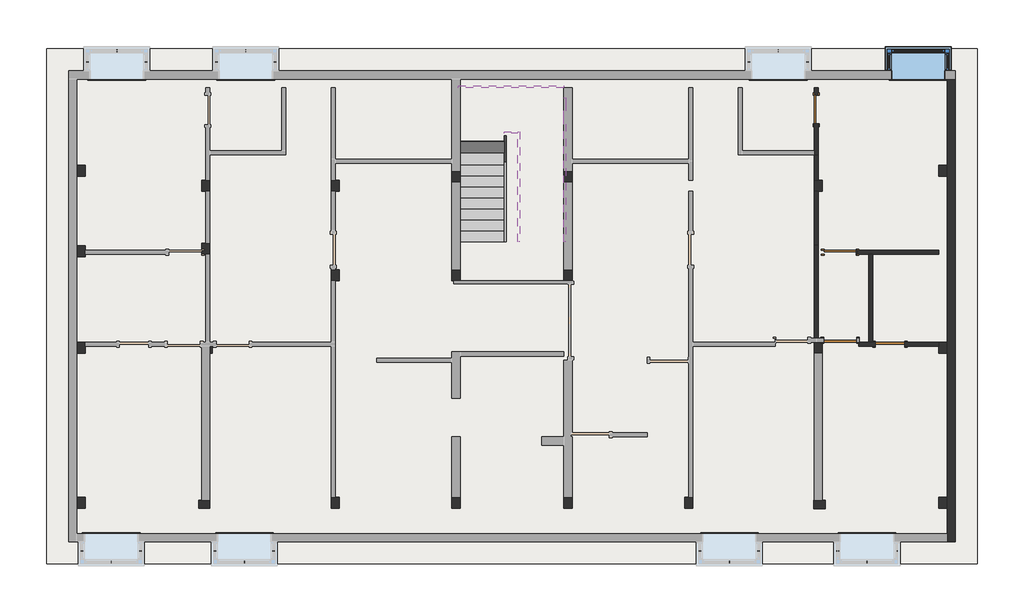
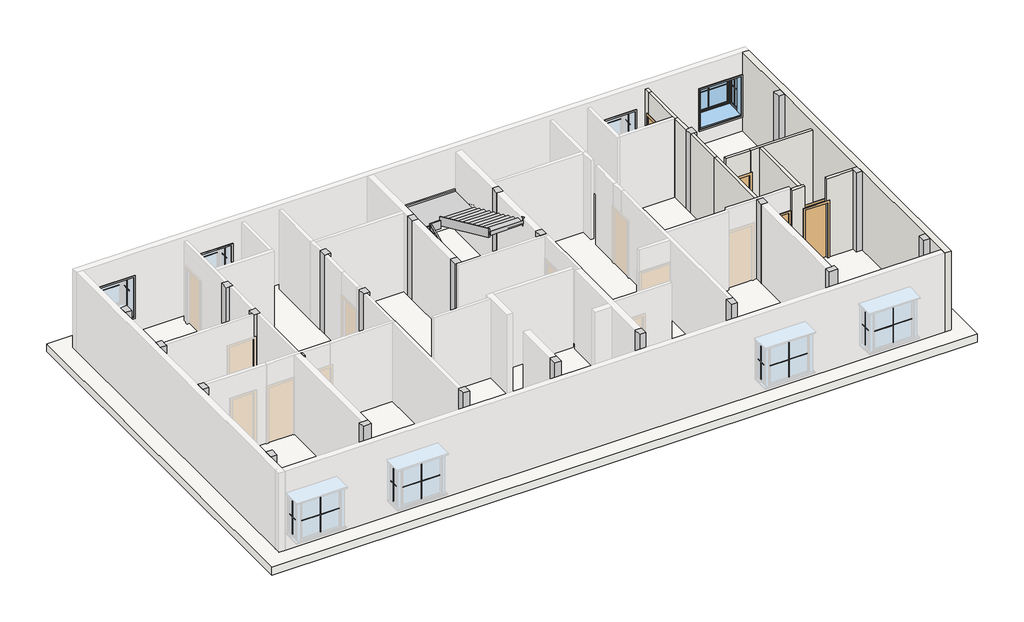
# One storey, part 2 of 2: 32 proxies, 24 columns, 11 walls, 6 members, 4 doors, 1 slab, 1 stair flight, 1 window.
"""IFC4 building model written with IfcOpenShell, lengths in millimetres."""

from ifc_helpers import new_model, si_unit, frame, origin, place, context, project, spatial, polyline, outline, extrude, faceted_brep, transform, mapped, element, save
from components import m_muntin_pattern_2x2_m_muntin_pattern_2x2_c1fd4460, m_muntin_pattern_2x2_m_muntin_pattern_2x2_777b163a, m_trim_window_interior_flat_picture_frame_44e8afef, column_efe9d5a4, door_1991e9a2, door_a431d384, door_82def9da, m_door_single_panel_3_x7_f8176753, stair_flight_1c36809e, window_19bbd869

model = new_model("IFC4")

# Units and contexts
model_context = context("Model", 3, world=origin())
ifc_project = project(units=[si_unit("LENGTHUNIT", "METRE", prefix="MILLI")], contexts=[model_context])

# Site, building, storey
site = spatial("IfcSite", under=ifc_project)
building = spatial("IfcBuilding", under=site)
storey = spatial("IfcBuildingStorey", under=building, Elevation=16002.0)

# Proxies
placement = place(None, origin())
m_muntin_pattern_2x2_m_muntin_pattern_2x2_shape = m_muntin_pattern_2x2_m_muntin_pattern_2x2_c1fd4460(model_context)
element("IfcBuildingElementProxy", 1, Name="M_Muntin Pattern_2x2 : M_Muntin Pattern_2x2", ObjectType="M_Muntin Pattern_2x2 : M_Muntin Pattern_2x2", at=placement, inside=storey, context=model_context, shape_type="MappedRepresentation", body=[
    mapped(m_muntin_pattern_2x2_m_muntin_pattern_2x2_shape, transform((-11500.7987957, -5499.9182661, 16722.65), x_axis=(-1.0, 0.0, 0.0), y_axis=(0.0, -1.0, 0.0), z_axis=(0.0, 0.0, 1.0))),
])
element("IfcBuildingElementProxy", 2, Name="M_Muntin Pattern_2x2 : M_Muntin Pattern_2x2", ObjectType="M_Muntin Pattern_2x2 : M_Muntin Pattern_2x2", at=placement, inside=storey, context=model_context, shape_type="MappedRepresentation", body=[
    mapped(m_muntin_pattern_2x2_m_muntin_pattern_2x2_shape, transform((-7819.250543, -5499.9182661, 16722.65), x_axis=(-1.0, 0.0, 0.0), y_axis=(0.0, -1.0, 0.0), z_axis=(0.0, 0.0, 1.0))),
])
element("IfcBuildingElementProxy", 3, Name="M_Muntin Pattern_2x2 : M_Muntin Pattern_2x2", ObjectType="M_Muntin Pattern_2x2 : M_Muntin Pattern_2x2", at=placement, inside=storey, context=model_context, shape_type="MappedRepresentation", body=[
    mapped(m_muntin_pattern_2x2_m_muntin_pattern_2x2_shape, transform((5599.7512082, -5499.9182661, 16722.65), x_axis=(-1.0, 0.0, 0.0), y_axis=(0.0, -1.0, 0.0), z_axis=(0.0, 0.0, 1.0))),
])
element("IfcBuildingElementProxy", 4, Name="M_Muntin Pattern_2x2 : M_Muntin Pattern_2x2", ObjectType="M_Muntin Pattern_2x2 : M_Muntin Pattern_2x2", at=placement, inside=storey, context=model_context, shape_type="MappedRepresentation", body=[
    mapped(m_muntin_pattern_2x2_m_muntin_pattern_2x2_shape, transform((9408.6146942, -5499.9182662, 16722.65), x_axis=(-1.0, 0.0, 0.0), y_axis=(0.0, -1.0, 0.0), z_axis=(0.0, 0.0, 1.0))),
])
element("IfcBuildingElementProxy", 5, Name="M_Muntin Pattern_2x2 : M_Muntin Pattern_2x2", ObjectType="M_Muntin Pattern_2x2 : M_Muntin Pattern_2x2", at=placement, inside=storey, context=model_context, shape_type="MappedRepresentation", body=[
    mapped(m_muntin_pattern_2x2_m_muntin_pattern_2x2_shape, transform((-11348.3987957, 8647.7317329, 16722.65), x_axis=(1.0, 0.0, 0.0), y_axis=(0.0, 1.0, 0.0), z_axis=(0.0, 0.0, 1.0))),
])
element("IfcBuildingElementProxy", 6, Name="M_Muntin Pattern_2x2 : M_Muntin Pattern_2x2", ObjectType="M_Muntin Pattern_2x2 : M_Muntin Pattern_2x2", at=placement, inside=storey, context=model_context, shape_type="MappedRepresentation", body=[
    mapped(m_muntin_pattern_2x2_m_muntin_pattern_2x2_shape, transform((-7779.6987993, 8647.7317329, 16722.65), x_axis=(1.0, 0.0, 0.0), y_axis=(0.0, 1.0, 0.0), z_axis=(0.0, 0.0, 1.0))),
])
element("IfcBuildingElementProxy", 7, Name="M_Muntin Pattern_2x2 : M_Muntin Pattern_2x2", ObjectType="M_Muntin Pattern_2x2 : M_Muntin Pattern_2x2", at=placement, inside=storey, context=model_context, shape_type="MappedRepresentation", body=[
    mapped(m_muntin_pattern_2x2_m_muntin_pattern_2x2_shape, transform((6952.301208, 8647.7317329, 16722.65), x_axis=(1.0, 0.0, 0.0), y_axis=(0.0, 1.0, 0.0), z_axis=(0.0, 0.0, 1.0))),
])
element("IfcBuildingElementProxy", 8, Name="M_Muntin Pattern_2x2 : M_Muntin Pattern_2x2", ObjectType="M_Muntin Pattern_2x2 : M_Muntin Pattern_2x2", at=placement, inside=storey, context=model_context, shape_type="MappedRepresentation", body=[
    mapped(m_muntin_pattern_2x2_m_muntin_pattern_2x2_shape, transform((10825.8012075, 8647.7317329, 16722.65), x_axis=(1.0, 0.0, 0.0), y_axis=(0.0, 1.0, 0.0), z_axis=(0.0, 0.0, 1.0))),
])
m_muntin_pattern_2x2_m_muntin_pattern_2x2_2_shape = m_muntin_pattern_2x2_m_muntin_pattern_2x2_777b163a(model_context)
element("IfcBuildingElementProxy", 9, Name="M_Muntin Pattern_2x2 : M_Muntin Pattern_2x2", ObjectType="M_Muntin Pattern_2x2 : M_Muntin Pattern_2x2", at=placement, inside=storey, context=model_context, shape_type="MappedRepresentation", body=[
    mapped(m_muntin_pattern_2x2_m_muntin_pattern_2x2_2_shape, transform((-10690.4737957, -5190.3932661, 16722.65), x_axis=(0.0, 1.0, 0.0), y_axis=(-1.0, 0.0, 0.0), z_axis=(0.0, 0.0, 1.0))),
])
element("IfcBuildingElementProxy", 10, Name="M_Muntin Pattern_2x2 : M_Muntin Pattern_2x2", ObjectType="M_Muntin Pattern_2x2 : M_Muntin Pattern_2x2", at=placement, inside=storey, context=model_context, shape_type="MappedRepresentation", body=[
    mapped(m_muntin_pattern_2x2_m_muntin_pattern_2x2_2_shape, transform((-12311.1237957, -5190.3932661, 16722.65), x_axis=(0.0, -1.0, 0.0), y_axis=(1.0, 0.0, 0.0), z_axis=(0.0, 0.0, 1.0))),
])
element("IfcBuildingElementProxy", 11, Name="M_Muntin Pattern_2x2 : M_Muntin Pattern_2x2", ObjectType="M_Muntin Pattern_2x2 : M_Muntin Pattern_2x2", at=placement, inside=storey, context=model_context, shape_type="MappedRepresentation", body=[
    mapped(m_muntin_pattern_2x2_m_muntin_pattern_2x2_2_shape, transform((-7008.925543, -5190.3932661, 16722.65), x_axis=(0.0, 1.0, 0.0), y_axis=(-1.0, 0.0, 0.0), z_axis=(0.0, 0.0, 1.0))),
])
element("IfcBuildingElementProxy", 12, Name="M_Muntin Pattern_2x2 : M_Muntin Pattern_2x2", ObjectType="M_Muntin Pattern_2x2 : M_Muntin Pattern_2x2", at=placement, inside=storey, context=model_context, shape_type="MappedRepresentation", body=[
    mapped(m_muntin_pattern_2x2_m_muntin_pattern_2x2_2_shape, transform((-8629.575543, -5190.3932661, 16722.65), x_axis=(0.0, -1.0, 0.0), y_axis=(1.0, 0.0, 0.0), z_axis=(0.0, 0.0, 1.0))),
])
element("IfcBuildingElementProxy", 13, Name="M_Muntin Pattern_2x2 : M_Muntin Pattern_2x2", ObjectType="M_Muntin Pattern_2x2 : M_Muntin Pattern_2x2", at=placement, inside=storey, context=model_context, shape_type="MappedRepresentation", body=[
    mapped(m_muntin_pattern_2x2_m_muntin_pattern_2x2_2_shape, transform((6410.0762082, -5190.3932661, 16722.65), x_axis=(0.0, 1.0, 0.0), y_axis=(-1.0, 0.0, 0.0), z_axis=(0.0, 0.0, 1.0))),
])
element("IfcBuildingElementProxy", 14, Name="M_Muntin Pattern_2x2 : M_Muntin Pattern_2x2", ObjectType="M_Muntin Pattern_2x2 : M_Muntin Pattern_2x2", at=placement, inside=storey, context=model_context, shape_type="MappedRepresentation", body=[
    mapped(m_muntin_pattern_2x2_m_muntin_pattern_2x2_2_shape, transform((4789.4262082, -5190.3932661, 16722.65), x_axis=(0.0, -1.0, 0.0), y_axis=(1.0, 0.0, 0.0), z_axis=(0.0, 0.0, 1.0))),
])
element("IfcBuildingElementProxy", 15, Name="M_Muntin Pattern_2x2 : M_Muntin Pattern_2x2", ObjectType="M_Muntin Pattern_2x2 : M_Muntin Pattern_2x2", at=placement, inside=storey, context=model_context, shape_type="MappedRepresentation", body=[
    mapped(m_muntin_pattern_2x2_m_muntin_pattern_2x2_2_shape, transform((10218.9396942, -5190.3932662, 16722.65), x_axis=(0.0, 1.0, 0.0), y_axis=(-1.0, 0.0, 0.0), z_axis=(0.0, 0.0, 1.0))),
])
element("IfcBuildingElementProxy", 16, Name="M_Muntin Pattern_2x2 : M_Muntin Pattern_2x2", ObjectType="M_Muntin Pattern_2x2 : M_Muntin Pattern_2x2", at=placement, inside=storey, context=model_context, shape_type="MappedRepresentation", body=[
    mapped(m_muntin_pattern_2x2_m_muntin_pattern_2x2_2_shape, transform((8598.2896942, -5190.3932661, 16722.65), x_axis=(0.0, -1.0, 0.0), y_axis=(1.0, 0.0, 0.0), z_axis=(0.0, 0.0, 1.0))),
])
element("IfcBuildingElementProxy", 17, Name="M_Muntin Pattern_2x2 : M_Muntin Pattern_2x2", ObjectType="M_Muntin Pattern_2x2 : M_Muntin Pattern_2x2", at=placement, inside=storey, context=model_context, shape_type="MappedRepresentation", body=[
    mapped(m_muntin_pattern_2x2_m_muntin_pattern_2x2_2_shape, transform((-12158.7237957, 8338.2067329, 16722.65), x_axis=(0.0, -1.0, 0.0), y_axis=(1.0, 0.0, 0.0), z_axis=(0.0, 0.0, 1.0))),
])
element("IfcBuildingElementProxy", 18, Name="M_Muntin Pattern_2x2 : M_Muntin Pattern_2x2", ObjectType="M_Muntin Pattern_2x2 : M_Muntin Pattern_2x2", at=placement, inside=storey, context=model_context, shape_type="MappedRepresentation", body=[
    mapped(m_muntin_pattern_2x2_m_muntin_pattern_2x2_2_shape, transform((-10538.0737957, 8338.2067329, 16722.65), x_axis=(0.0, 1.0, 0.0), y_axis=(-1.0, 0.0, 0.0), z_axis=(0.0, 0.0, 1.0))),
])
element("IfcBuildingElementProxy", 19, Name="M_Muntin Pattern_2x2 : M_Muntin Pattern_2x2", ObjectType="M_Muntin Pattern_2x2 : M_Muntin Pattern_2x2", at=placement, inside=storey, context=model_context, shape_type="MappedRepresentation", body=[
    mapped(m_muntin_pattern_2x2_m_muntin_pattern_2x2_2_shape, transform((-8590.0237993, 8338.2067329, 16722.65), x_axis=(0.0, -1.0, 0.0), y_axis=(1.0, 0.0, 0.0), z_axis=(0.0, 0.0, 1.0))),
])
element("IfcBuildingElementProxy", 20, Name="M_Muntin Pattern_2x2 : M_Muntin Pattern_2x2", ObjectType="M_Muntin Pattern_2x2 : M_Muntin Pattern_2x2", at=placement, inside=storey, context=model_context, shape_type="MappedRepresentation", body=[
    mapped(m_muntin_pattern_2x2_m_muntin_pattern_2x2_2_shape, transform((-6969.3737993, 8338.2067329, 16722.65), x_axis=(0.0, 1.0, 0.0), y_axis=(-1.0, 0.0, 0.0), z_axis=(0.0, 0.0, 1.0))),
])
element("IfcBuildingElementProxy", 21, Name="M_Muntin Pattern_2x2 : M_Muntin Pattern_2x2", ObjectType="M_Muntin Pattern_2x2 : M_Muntin Pattern_2x2", at=placement, inside=storey, context=model_context, shape_type="MappedRepresentation", body=[
    mapped(m_muntin_pattern_2x2_m_muntin_pattern_2x2_2_shape, transform((6141.976208, 8338.2067329, 16722.65), x_axis=(0.0, -1.0, 0.0), y_axis=(1.0, 0.0, 0.0), z_axis=(0.0, 0.0, 1.0))),
])
element("IfcBuildingElementProxy", 22, Name="M_Muntin Pattern_2x2 : M_Muntin Pattern_2x2", ObjectType="M_Muntin Pattern_2x2 : M_Muntin Pattern_2x2", at=placement, inside=storey, context=model_context, shape_type="MappedRepresentation", body=[
    mapped(m_muntin_pattern_2x2_m_muntin_pattern_2x2_2_shape, transform((7762.626208, 8338.2067329, 16722.65), x_axis=(0.0, 1.0, 0.0), y_axis=(-1.0, 0.0, 0.0), z_axis=(0.0, 0.0, 1.0))),
])
element("IfcBuildingElementProxy", 23, Name="M_Muntin Pattern_2x2 : M_Muntin Pattern_2x2", ObjectType="M_Muntin Pattern_2x2 : M_Muntin Pattern_2x2", at=placement, inside=storey, context=model_context, shape_type="MappedRepresentation", body=[
    mapped(m_muntin_pattern_2x2_m_muntin_pattern_2x2_2_shape, transform((10015.4762075, 8338.2067329, 16722.65), x_axis=(0.0, -1.0, 0.0), y_axis=(1.0, 0.0, 0.0), z_axis=(0.0, 0.0, 1.0))),
])
element("IfcBuildingElementProxy", 24, Name="M_Muntin Pattern_2x2 : M_Muntin Pattern_2x2", ObjectType="M_Muntin Pattern_2x2 : M_Muntin Pattern_2x2", at=placement, inside=storey, context=model_context, shape_type="MappedRepresentation", body=[
    mapped(m_muntin_pattern_2x2_m_muntin_pattern_2x2_2_shape, transform((11636.1262075, 8338.2067329, 16722.65), x_axis=(0.0, 1.0, 0.0), y_axis=(-1.0, 0.0, 0.0), z_axis=(0.0, 0.0, 1.0))),
])
m_trim_window_interior_flat_picture_frame_shape = m_trim_window_interior_flat_picture_frame_44e8afef(model_context)
element("IfcBuildingElementProxy", 25, Name="M_Trim-Window-Interior-Flat : Picture Frame", ObjectType="M_Trim-Window-Interior-Flat : Picture Frame", at=placement, inside=storey, context=model_context, shape_type="MappedRepresentation", body=[
    mapped(m_trim_window_interior_flat_picture_frame_shape, transform((-11500.7987957, -4712.5932661, 18152.8), x_axis=(-1.0, 0.0, 0.0), y_axis=(0.0, 0.0, 1.0), z_axis=(0.0, 1.0, 0.0))),
])
element("IfcBuildingElementProxy", 26, Name="M_Trim-Window-Interior-Flat : Picture Frame", ObjectType="M_Trim-Window-Interior-Flat : Picture Frame", at=placement, inside=storey, context=model_context, shape_type="MappedRepresentation", body=[
    mapped(m_trim_window_interior_flat_picture_frame_shape, transform((-7819.250543, -4712.5932661, 18152.8), x_axis=(-1.0, 0.0, 0.0), y_axis=(0.0, 0.0, 1.0), z_axis=(0.0, 1.0, 0.0))),
])
element("IfcBuildingElementProxy", 27, Name="M_Trim-Window-Interior-Flat : Picture Frame", ObjectType="M_Trim-Window-Interior-Flat : Picture Frame", at=placement, inside=storey, context=model_context, shape_type="MappedRepresentation", body=[
    mapped(m_trim_window_interior_flat_picture_frame_shape, transform((5599.7512082, -4712.5932661, 18152.8), x_axis=(-1.0, 0.0, 0.0), y_axis=(0.0, 0.0, 1.0), z_axis=(0.0, 1.0, 0.0))),
])
element("IfcBuildingElementProxy", 28, Name="M_Trim-Window-Interior-Flat : Picture Frame", ObjectType="M_Trim-Window-Interior-Flat : Picture Frame", at=placement, inside=storey, context=model_context, shape_type="MappedRepresentation", body=[
    mapped(m_trim_window_interior_flat_picture_frame_shape, transform((9408.6146942, -4712.5932661, 18152.8), x_axis=(-1.0, 0.0, 0.0), y_axis=(0.0, 0.0, 1.0), z_axis=(0.0, 1.0, 0.0))),
])
element("IfcBuildingElementProxy", 29, Name="M_Trim-Window-Interior-Flat : Picture Frame", ObjectType="M_Trim-Window-Interior-Flat : Picture Frame", at=placement, inside=storey, context=model_context, shape_type="MappedRepresentation", body=[
    mapped(m_trim_window_interior_flat_picture_frame_shape, transform((-11348.3987957, 7860.4067329, 18152.8), x_axis=(1.0, 0.0, 0.0), y_axis=(0.0, 0.0, 1.0), z_axis=(0.0, -1.0, 0.0))),
])
element("IfcBuildingElementProxy", 30, Name="M_Trim-Window-Interior-Flat : Picture Frame", ObjectType="M_Trim-Window-Interior-Flat : Picture Frame", at=placement, inside=storey, context=model_context, shape_type="MappedRepresentation", body=[
    mapped(m_trim_window_interior_flat_picture_frame_shape, transform((-7779.6987993, 7860.4067329, 18152.8), x_axis=(1.0, 0.0, 0.0), y_axis=(0.0, 0.0, 1.0), z_axis=(0.0, -1.0, 0.0))),
])
element("IfcBuildingElementProxy", 31, Name="M_Trim-Window-Interior-Flat : Picture Frame", ObjectType="M_Trim-Window-Interior-Flat : Picture Frame", at=placement, inside=storey, context=model_context, shape_type="MappedRepresentation", body=[
    mapped(m_trim_window_interior_flat_picture_frame_shape, transform((6952.301208, 7860.4067329, 18152.8), x_axis=(1.0, 0.0, 0.0), y_axis=(0.0, 0.0, 1.0), z_axis=(0.0, -1.0, 0.0))),
])
element("IfcBuildingElementProxy", 32, Name="M_Trim-Window-Interior-Flat : Picture Frame", ObjectType="M_Trim-Window-Interior-Flat : Picture Frame", at=placement, inside=storey, context=model_context, shape_type="MappedRepresentation", body=[
    mapped(m_trim_window_interior_flat_picture_frame_shape, transform((10825.8012075, 7860.4067329, 18152.8), x_axis=(1.0, 0.0, 0.0), y_axis=(0.0, 0.0, 1.0), z_axis=(0.0, -1.0, 0.0))),
])

# Columns
element("IfcColumn", 33, ObjectType="Rectangular Column : 1'X 9\"", at=placement, inside=storey, context=model_context, shape_type="SweptSolid", body=[
    extrude(outline(polyline([(-12224.6987957, -3709.2932671), (-12224.6987957, -4014.0932671), (-12453.2987957, -4014.0932671), (-12453.2987957, -3709.2932671), (-12224.6987957, -3709.2932671)])), frame((0.0, 0.0, 16002.0), z_axis=(0.0, 0.0, 1.0), x_axis=(1.0, 0.0, 0.0)), (0.0, 0.0, 1.0), 3048.0),
])
element("IfcColumn", 34, ObjectType="Rectangular Column : 1'X 9\"", at=placement, inside=storey, context=model_context, shape_type="SweptSolid", body=[
    extrude(outline(polyline([(-12224.6987957, 583.3067334), (-12224.6987957, 278.5067334), (-12453.2987957, 278.5067334), (-12453.2987957, 583.3067334), (-12224.6987957, 583.3067334)])), frame((0.0, 0.0, 16002.0), z_axis=(0.0, 0.0, 1.0), x_axis=(1.0, 0.0, 0.0)), (0.0, 0.0, 1.0), 3048.0),
])
element("IfcColumn", 35, ObjectType="Rectangular Column : 1'X 9\"", at=placement, inside=storey, context=model_context, shape_type="SweptSolid", body=[
    extrude(outline(polyline([(-12224.6987957, 3256.6567332), (-12224.6987957, 2951.8567332), (-12453.2987957, 2951.8567332), (-12453.2987957, 3256.6567332), (-12224.6987957, 3256.6567332)])), frame((0.0, 0.0, 16002.0), z_axis=(0.0, 0.0, 1.0), x_axis=(1.0, 0.0, 0.0)), (0.0, 0.0, 1.0), 3048.0),
])
element("IfcColumn", 36, ObjectType="Rectangular Column : 1'X 9\"", at=placement, inside=storey, context=model_context, shape_type="Brep", body=[
    faceted_brep([(-8770.2987992, 5066.406733, 16002.0), (-8770.2987992, 4761.606733, 16002.0), (-8884.5987992, 4761.606733, 16002.0), (-8998.8987992, 4761.606733, 16002.0), (-8998.8987992, 5066.406733, 16002.0), (-8884.5987992, 5066.406733, 16002.0), (-8770.2987992, 5066.406733, 19050.0), (-8770.2987992, 4761.606733, 19050.0), (-8884.5987992, 4761.606733, 19050.0), (-8998.8987992, 4761.606733, 19050.0), (-8998.8987992, 5066.406733, 19050.0), (-8884.5987992, 5066.406733, 19050.0)], [[[0, 1, 2, 3, 4, 5]], [[6, 7, 1, 0]], [[7, 8, 9, 3, 2, 1]], [[9, 10, 4, 3]], [[10, 11, 6, 0, 5, 4]], [[6, 11, 10, 9, 8, 7]]]),
])
element("IfcColumn", 37, ObjectType="Rectangular Column : 1'X 9\"", at=placement, inside=storey, context=model_context, shape_type="Brep", body=[
    faceted_brep([(-8770.2987992, 3326.5067332, 16002.0), (-8770.2987992, 3021.7067332, 16002.0), (-8884.598796, 3021.7067332, 16002.0), (-8998.8987992, 3021.7067332, 16002.0), (-8998.8987992, 3326.5067332, 16002.0), (-8884.5987992, 3326.5067332, 16002.0), (-8770.2987992, 3326.5067332, 19050.0), (-8770.2987992, 3021.7067332, 19050.0), (-8884.598796, 3021.7067332, 19050.0), (-8998.8987992, 3021.7067332, 19050.0), (-8998.8987992, 3326.5067332, 19050.0), (-8884.5987992, 3326.5067332, 19050.0)], [[[0, 1, 2, 3, 4, 5]], [[6, 7, 1, 0]], [[7, 8, 9, 3, 2, 1]], [[9, 10, 4, 3]], [[10, 11, 6, 0, 5, 4]], [[6, 11, 10, 9, 8, 7]]]),
])
element("IfcColumn", 38, ObjectType="Rectangular Column : 1'X 9\"", at=placement, inside=storey, context=model_context, shape_type="SweptSolid", body=[
    extrude(outline(polyline([(-8713.148796, 278.5067334), (-8771.750543, 278.5067334), (-8771.750543, 469.0067334), (-8713.148796, 469.0067334), (-8713.148796, 278.5067334)])), frame((0.0, 0.0, 16002.0), z_axis=(0.0, 0.0, 1.0), x_axis=(1.0, 0.0, 0.0)), (0.0, 0.0, 1.0), 3048.0),
])
element("IfcColumn", 39, ObjectType="Rectangular Column : 1'X 9\"", at=placement, inside=storey, context=model_context, shape_type="Brep", body=[
    faceted_brep([(-5188.8987995, 5066.406733, 16002.0), (-5188.8987995, 4761.606733, 16002.0), (-5303.1987995, 4761.606733, 16002.0), (-5417.4987995, 4761.606733, 16002.0), (-5417.4987995, 5066.406733, 16002.0), (-5303.1987995, 5066.406733, 16002.0), (-5188.8987995, 5066.406733, 19050.0), (-5188.8987995, 4761.606733, 19050.0), (-5303.1987995, 4761.606733, 19050.0), (-5417.4987995, 4761.606733, 19050.0), (-5417.4987995, 5066.406733, 19050.0), (-5303.1987995, 5066.406733, 19050.0)], [[[0, 1, 2, 3, 4, 5]], [[6, 7, 1, 0]], [[7, 8, 9, 3, 2, 1]], [[9, 10, 4, 3]], [[10, 11, 6, 0, 5, 4]], [[6, 11, 10, 9, 8, 7]]]),
])
element("IfcColumn", 40, ObjectType="Rectangular Column : 1'X 9\"", at=placement, inside=storey, context=model_context, shape_type="Brep", body=[
    faceted_brep([(-5188.8987995, 2589.9067802, 16002.0), (-5188.8987995, 2285.1067802, 16002.0), (-5303.1987995, 2285.1067802, 16002.0), (-5417.4987995, 2285.1067802, 16002.0), (-5417.4987995, 2589.9067802, 16002.0), (-5303.1987995, 2589.9067802, 16002.0), (-5188.8987995, 2589.9067802, 19050.0), (-5188.8987995, 2285.1067802, 19050.0), (-5303.1987995, 2285.1067802, 19050.0), (-5417.4987995, 2285.1067802, 19050.0), (-5417.4987995, 2589.9067802, 19050.0), (-5303.1987995, 2589.9067802, 19050.0)], [[[0, 1, 2, 3, 4, 5]], [[6, 7, 1, 0]], [[7, 8, 9, 3, 2, 1]], [[9, 10, 4, 3]], [[10, 11, 6, 0, 5, 4]], [[6, 11, 10, 9, 8, 7]]]),
])
element("IfcColumn", 41, ObjectType="Rectangular Column : 1'X 9\"", at=placement, inside=storey, context=model_context, shape_type="Brep", body=[
    faceted_brep([(-5188.8987963, -3709.2932193, 16002.0), (-5188.8987963, -4014.0932193, 16002.0), (-5417.4987963, -4014.0932193, 16002.0), (-5417.4987963, -3709.2932193, 16002.0), (-5303.1987995, -3709.2932193, 16002.0), (-5188.8987963, -3709.2932193, 19050.0), (-5188.8987963, -4014.0932193, 19050.0), (-5417.4987963, -4014.0932193, 19050.0), (-5417.4987963, -3709.2932193, 19050.0), (-5303.1987995, -3709.2932193, 19050.0)], [[[0, 1, 2, 3, 4]], [[5, 6, 1, 0]], [[6, 7, 2, 1]], [[7, 8, 3, 2]], [[8, 9, 5, 0, 4, 3]], [[5, 9, 8, 7, 6]]]),
])
element("IfcColumn", 42, ObjectType="Rectangular Column : 1'X 9\"", at=placement, inside=storey, context=model_context, shape_type="SweptSolid", body=[
    extrude(outline(polyline([(1250.0012085, -3709.2932193), (1250.0012085, -4014.0932193), (1021.4012085, -4014.0932193), (1021.4012085, -3709.2932193), (1250.0012085, -3709.2932193)])), frame((0.0, 0.0, 16002.0), z_axis=(0.0, 0.0, 1.0), x_axis=(1.0, 0.0, 0.0)), (0.0, 0.0, 1.0), 3048.0),
])
element("IfcColumn", 43, ObjectType="Rectangular Column : 1'X 9\"", at=placement, inside=storey, context=model_context, shape_type="Brep", body=[
    faceted_brep([(4590.1012082, -3709.2932193, 16002.0), (4590.1012082, -4014.0932193, 16002.0), (4361.5012082, -4014.0932193, 16002.0), (4361.5012082, -3709.2932193, 16002.0), (4475.8012082, -3709.2932193, 16002.0), (4590.1012082, -3709.2932193, 19050.0), (4590.1012082, -4014.0932193, 19050.0), (4361.5012082, -4014.0932193, 19050.0), (4361.5012082, -3709.2932193, 19050.0), (4475.8012082, -3709.2932193, 19050.0)], [[[0, 1, 2, 3, 4]], [[5, 6, 1, 0]], [[6, 7, 2, 1]], [[7, 8, 3, 2]], [[8, 9, 5, 0, 4, 3]], [[5, 9, 8, 7, 6]]]),
])
element("IfcColumn", 44, ObjectType="Rectangular Column : 1'X 9\"", at=placement, inside=storey, context=model_context, shape_type="SweptSolid", body=[
    extrude(outline(polyline([(11625.9012075, -3709.2932671), (11625.9012075, -4014.0932671), (11397.3012075, -4014.0932671), (11397.3012075, -3709.2932671), (11625.9012075, -3709.2932671)])), frame((0.0, 0.0, 16002.0), z_axis=(0.0, 0.0, 1.0), x_axis=(1.0, 0.0, 0.0)), (0.0, 0.0, 1.0), 3048.0),
])
element("IfcColumn", 45, ObjectType="Rectangular Column : 1'X 9\"", at=placement, inside=storey, context=model_context, shape_type="Brep", body=[
    faceted_brep([(11625.9012075, 583.3067295, 16002.0), (11625.9012075, 278.5067295, 16002.0), (11397.3012075, 278.5067295, 16002.0), (11397.3012075, 469.0067295, 16002.0), (11397.3012075, 583.3067295, 16002.0), (11625.9012075, 583.3067295, 19050.0), (11625.9012075, 278.5067295, 19050.0), (11397.3012075, 278.5067295, 19050.0), (11397.3012075, 469.0067295, 19050.0), (11397.3012075, 583.3067295, 19050.0)], [[[0, 1, 2, 3, 4]], [[5, 6, 1, 0]], [[6, 7, 2, 1]], [[7, 8, 9, 4, 3, 2]], [[9, 5, 0, 4]], [[5, 9, 8, 7, 6]]]),
])
element("IfcColumn", 46, ObjectType="Rectangular Column : 1'X 9\"", at=placement, inside=storey, context=model_context, shape_type="SweptSolid", body=[
    extrude(outline(polyline([(11625.9012075, 5479.1567329), (11625.9012075, 5174.3567329), (11397.3012075, 5174.3567329), (11397.3012075, 5479.1567329), (11625.9012075, 5479.1567329)])), frame((0.0, 0.0, 16002.0), z_axis=(0.0, 0.0, 1.0), x_axis=(1.0, 0.0, 0.0)), (0.0, 0.0, 1.0), 3048.0),
])
element("IfcColumn", 47, ObjectType="Rectangular Column : 1'X 9\"", at=placement, inside=storey, context=model_context, shape_type="Brep", body=[
    faceted_brep([(8172.5040565, 5065.4824989, 16002.0), (8172.5040565, 4760.6824989, 16002.0), (8057.2012047, 4760.6824989, 16002.0), (7943.9040565, 4760.6824989, 16002.0), (7943.9040565, 5065.4824989, 16002.0), (8058.2040565, 5065.4824989, 16002.0), (8172.5040565, 5065.4824989, 19050.0), (8172.5040565, 4760.6824989, 19050.0), (8057.2012047, 4760.6824989, 19050.0), (7943.9040565, 4760.6824989, 19050.0), (7943.9040565, 5065.4824989, 19050.0), (8058.2040565, 5065.4824989, 19050.0)], [[[0, 1, 2, 3, 4, 5]], [[6, 7, 1, 0]], [[7, 8, 9, 3, 2, 1]], [[9, 10, 4, 3]], [[10, 11, 6, 0, 5, 4]], [[6, 11, 10, 9, 8, 7]]]),
])
element("IfcColumn", 48, ObjectType="Rectangular Column : 1'X 9\"", at=placement, inside=storey, context=model_context, shape_type="Brep", body=[
    faceted_brep([(8171.5012047, 583.3067334, 16002.0), (8171.5012047, 278.5067334, 16002.0), (7942.9012047, 278.5067334, 16002.0), (7942.9012047, 583.3067334, 16002.0), (8000.0512079, 583.3067334, 16002.0), (8171.5012047, 583.3067334, 19050.0), (8171.5012047, 278.5067334, 19050.0), (7942.9012047, 278.5067334, 19050.0), (7942.9012047, 583.3067334, 19050.0), (8000.0512079, 583.3067334, 19050.0)], [[[0, 1, 2, 3, 4]], [[5, 6, 1, 0]], [[6, 7, 2, 1]], [[7, 8, 3, 2]], [[8, 9, 5, 0, 4, 3]], [[5, 9, 8, 7, 6]]]),
])
element("IfcColumn", 49, ObjectType="Rectangular Column : 1'X 9\"", at=placement, inside=storey, context=model_context, shape_type="Brep", body=[
    faceted_brep([(-9076.550543, -3785.4932196, 16002.0), (-9000.350543, -3785.4932196, 16002.0), (-8771.750543, -3785.4932196, 16002.0), (-8771.750543, -4014.0932196, 16002.0), (-9076.550543, -4014.0932196, 16002.0), (-9076.550543, -3785.4932196, 19050.0), (-9000.350543, -3785.4932196, 19050.0), (-8771.750543, -3785.4932196, 19050.0), (-8771.750543, -4014.0932196, 19050.0), (-9076.550543, -4014.0932196, 19050.0)], [[[0, 1, 2, 3, 4]], [[5, 6, 7, 2, 1, 0]], [[7, 8, 3, 2]], [[8, 9, 4, 3]], [[9, 5, 0, 4]], [[5, 9, 8, 7, 6]]]),
])
element("IfcColumn", 50, ObjectType="Rectangular Column : 1'X 9\"", at=placement, inside=storey, context=model_context, shape_type="SweptSolid", body=[
    extrude(outline(polyline([(-12453.2987957, 5174.3567339), (-12453.2987957, 5479.1567339), (-12224.6987957, 5479.1567339), (-12224.6987957, 5174.3567339), (-12453.2987957, 5174.3567339)])), frame((0.0, 0.0, 16002.0), z_axis=(0.0, 0.0, 1.0), x_axis=(1.0, 0.0, 0.0)), (0.0, 0.0, 1.0), 3048.0),
])
element("IfcColumn", 51, ObjectType="Rectangular Column : 1'X 9\"", at=placement, inside=storey, context=model_context, shape_type="SweptSolid", body=[
    extrude(outline(polyline([(-1845.5417538, 5320.4067329), (-1845.5417538, 5015.6067329), (-2074.1417538, 5015.6067329), (-2074.1417538, 5320.4067329), (-1845.5417538, 5320.4067329)])), frame((0.0, 0.0, 16002.0), z_axis=(0.0, 0.0, 1.0), x_axis=(1.0, 0.0, 0.0)), (0.0, 0.0, 1.0), 3048.0),
])
element("IfcColumn", 52, ObjectType="Rectangular Column : 1'X 9\"", at=placement, inside=storey, context=model_context, shape_type="SweptSolid", body=[
    extrude(outline(polyline([(1250.0012085, 5320.4067329), (1250.0012085, 5015.6067329), (1021.4012085, 5015.6067329), (1021.4012085, 5320.4067329), (1250.0012085, 5320.4067329)])), frame((0.0, 0.0, 16002.0), z_axis=(0.0, 0.0, 1.0), x_axis=(1.0, 0.0, 0.0)), (0.0, 0.0, 1.0), 3048.0),
])
element("IfcColumn", 53, ObjectType="Rectangular Column : 1'X 9\"", at=placement, inside=storey, context=model_context, shape_type="Brep", body=[
    faceted_brep([(-1845.5417538, 2589.906774, 16002.0), (-1845.5417538, 2285.106774, 16002.0), (-2020.2487998, 2285.106774, 16002.0), (-2074.1417538, 2285.106774, 16002.0), (-2074.1417538, 2589.906774, 16002.0), (-1845.5417538, 2589.906774, 19050.0), (-1845.5417538, 2285.106774, 19050.0), (-2020.2487998, 2285.106774, 19050.0), (-2074.1417538, 2285.106774, 19050.0), (-2074.1417538, 2589.906774, 19050.0)], [[[0, 1, 2, 3, 4]], [[5, 6, 1, 0]], [[6, 7, 8, 3, 2, 1]], [[8, 9, 4, 3]], [[9, 5, 0, 4]], [[5, 9, 8, 7, 6]]]),
])
element("IfcColumn", 54, ObjectType="Rectangular Column : 1'X 9\"", at=placement, inside=storey, context=model_context, shape_type="Brep", body=[
    faceted_brep([(1253.2582462, 2589.9067742, 16002.0), (1253.2582462, 2285.1067742, 16002.0), (1024.6582462, 2285.1067742, 16002.0), (1024.6582462, 2589.9067742, 16002.0), (1250.0012085, 2589.9067742, 16002.0), (1253.2582462, 2589.9067742, 19050.0), (1253.2582462, 2285.1067742, 19050.0), (1024.6582462, 2285.1067742, 19050.0), (1024.6582462, 2589.9067742, 19050.0), (1250.0012085, 2589.9067742, 19050.0)], [[[0, 1, 2, 3, 4]], [[5, 6, 1, 0]], [[6, 7, 2, 1]], [[7, 8, 3, 2]], [[8, 9, 5, 0, 4, 3]], [[5, 9, 8, 7, 6]]]),
])
element("IfcColumn", 55, ObjectType="Rectangular Column : 1'X 9\"", at=placement, inside=storey, context=model_context, shape_type="SweptSolid", body=[
    extrude(outline(polyline([(-1848.7987998, -3709.2932663), (-1848.7987998, -4014.0932663), (-2077.3987998, -4014.0932663), (-2077.3987998, -3709.2932663), (-1848.7987998, -3709.2932663)])), frame((0.0, 0.0, 16002.0), z_axis=(0.0, 0.0, 1.0), x_axis=(1.0, 0.0, 0.0)), (0.0, 0.0, 1.0), 3048.0),
])
column_shape = column_efe9d5a4(model_context)
element("IfcColumn", 56, ObjectType="Rectangular Column : 1'X 9\"", at=placement, inside=storey, context=model_context, shape_type="MappedRepresentation", body=[
    mapped(column_shape, transform((8094.1646942, -3901.6914801, 0.0), x_axis=(0.0, 1.0, 0.0), y_axis=(-1.0, 0.0, 0.0), z_axis=(0.0, 0.0, 1.0))),
])

# Doors
door_shape = door_1991e9a2(model_context)
element("IfcDoor", 57, ObjectType="M_Door-Single-Panel : 2'11\"X7' 3", at=placement, inside=storey, context=model_context, shape_type="MappedRepresentation", body=[
    mapped(door_shape, transform((8664.274939, 3078.8567332, 16002.0), x_axis=(-1.0, 0.0, 0.0), y_axis=(0.0, -1.0, 0.0), z_axis=(0.0, 0.0, 1.0))),
])
door_2_shape = door_a431d384(model_context)
element("IfcDoor", 58, ObjectType="M_Door-Single-Panel : 2'7\"X7' 2", at=placement, inside=storey, context=model_context, shape_type="MappedRepresentation", body=[
    mapped(door_2_shape, transform((8000.0512079, 7021.3751452, 16002.0), x_axis=(0.0, 1.0, 0.0), y_axis=(-1.0, 0.0, 0.0), z_axis=(0.0, 0.0, 1.0))),
])
door_3_shape = door_82def9da(model_context)
element("IfcDoor", 59, ObjectType="M_Door-Single-Panel : 2'8\"X7'", at=placement, inside=storey, context=model_context, shape_type="MappedRepresentation", body=[
    mapped(door_3_shape, transform((10046.0486694, 526.1567295, 16002.0), x_axis=(-1.0, 0.0, 0.0), y_axis=(0.0, -1.0, 0.0), z_axis=(0.0, 0.0, 1.0))),
])
m_door_single_panel_3_x7_shape = m_door_single_panel_3_x7_f8176753(model_context)
element("IfcDoor", 60, ObjectType="M_Door-Single-Panel : 3'X7'", at=placement, inside=storey, context=model_context, shape_type="MappedRepresentation", body=[
    mapped(m_door_single_panel_3_x7_shape, transform((8666.8012079, 640.4567334, 16002.0), x_axis=(-1.0, 0.0, 0.0), y_axis=(0.0, -1.0, 0.0), z_axis=(0.0, 0.0, 1.0))),
])

# Members
element("IfcMember", 61, ObjectType="Stringer - 2\" Width", at=placement, inside=storey, context=model_context, shape_type="SweptSolid", body=[
    extrude(outline(polyline([(3364.6067329, 16002.0), (3364.6067329, 16201.8262721), (6445.4289342, 17602.2), (7182.0114168, 17602.2), (3661.5714168, 16002.0), (3364.6067329, 16002.0)])), frame((-1896.3417538, 0.0, 0.0), z_axis=(1.0, 0.0, 0.0), x_axis=(0.0, 1.0, 0.0)), (0.0, 0.0, 1.0), 50.8),
])
element("IfcMember", 62, ObjectType="Stringer - 2\" Width", at=placement, inside=storey, context=model_context, shape_type="SweptSolid", body=[
    extrude(outline(polyline([(-1896.3417538, 7631.8067329), (-1896.3417538, 7682.6067329), (1021.4012085, 7682.6067329), (1021.4012085, 7631.8067329), (-1896.3417538, 7631.8067329)])), frame((0.0, 0.0, 17297.4), z_axis=(0.0, 0.0, 1.0), x_axis=(1.0, 0.0, 0.0)), (0.0, 0.0, 1.0), 304.8),
])
element("IfcMember", 63, ObjectType="Stringer - 2\" Width", at=placement, inside=storey, context=model_context, shape_type="SweptSolid", body=[
    extrude(outline(polyline([(6618.562049, 17297.4), (3364.6067329, 18776.4705982), (3364.6067329, 19111.2808176), (7355.1445316, 17297.4), (6618.562049, 17297.4)])), frame((1021.4012085, 0.0, 0.0), z_axis=(1.0, 0.0, 0.0), x_axis=(0.0, 1.0, 0.0)), (0.0, 0.0, 1.0), 50.8),
])
element("IfcMember", 64, ObjectType="Stringer - 2\" Width", at=placement, inside=storey, context=model_context, shape_type="SweptSolid", body=[
    extrude(outline(polyline([(3364.6067329, 16002.0), (3364.6067329, 16201.8262721), (6361.8067329, 17564.1899085), (6361.8067329, 17229.3796892), (3661.5714168, 16002.0), (3364.6067329, 16002.0)])), frame((-629.5987998, 0.0, 0.0), z_axis=(1.0, 0.0, 0.0), x_axis=(0.0, 1.0, 0.0)), (0.0, 0.0, 1.0), 50.8),
])
element("IfcMember", 65, ObjectType="Stringer - 2\" Width", at=placement, inside=storey, context=model_context, shape_type="SweptSolid", body=[
    extrude(outline(polyline([(-629.5987998, 6361.8067329), (-629.5987998, 6412.6067329), (-248.5987915, 6412.6067329), (-248.5987915, 6361.8067329), (-629.5987998, 6361.8067329)])), frame((0.0, 0.0, 17297.4), z_axis=(0.0, 0.0, 1.0), x_axis=(1.0, 0.0, 0.0)), (0.0, 0.0, 1.0), 304.8),
])
element("IfcMember", 66, ObjectType="Stringer - 2\" Width", at=placement, inside=storey, context=model_context, shape_type="SweptSolid", body=[
    extrude(outline(polyline([(6412.6067329, 17725.8262721), (6412.6067329, 17391.0160528), (3364.6067329, 18776.4705982), (3364.6067329, 19111.2808176), (6412.6067329, 17725.8262721)])), frame((-248.5987915, 0.0, 0.0), z_axis=(1.0, 0.0, 0.0), x_axis=(0.0, 1.0, 0.0)), (0.0, 0.0, 1.0), 50.8),
])

# Slab
element("IfcSlab", 67, ObjectType="Generic - 12\"", at=placement, inside=storey, context=model_context, shape_type="SweptSolid", body=[
    extrude(outline(polyline([(12464.1012075, 8698.6067329), (12464.1012075, -5550.7932662), (-13291.4987957, -5550.7932662), (-13291.4987957, 8698.6067329), (12464.1012075, 8698.6067329)])), frame((0.0, 0.0, 15697.2), z_axis=(0.0, 0.0, 1.0), x_axis=(1.0, 0.0, 0.0)), (0.0, 0.0, 1.0), 304.8),
])

# Stair flight
stair_flight_shape = stair_flight_1c36809e(model_context)
element("IfcStairFlight", 68, ObjectType="2\" Tread 1\" Nosing 1/4\" Riser", at=placement, inside=storey, context=model_context, shape_type="MappedRepresentation", body=[
    mapped(stair_flight_shape, transform((0.0, 0.0, 0.0), x_axis=(1.0, 0.0, 0.0), y_axis=(0.0, 1.0, 0.0), z_axis=(0.0, 0.0, 1.0))),
])

# Walls
element("IfcWall", 69, ObjectType="4.5\"", at=placement, inside=storey, context=model_context, shape_type="SweptSolid", body=[
    extrude(outline(polyline([(16002.0, 9131.6486701), (19050.0, 9131.6486701), (19050.0, 8245.174939), (18135.6, 8245.174939), (18135.6, 9108.774939), (16002.0, 9108.774939), (16002.0, 9131.6486701)])), frame((0.0, 3021.7067332, 0.0), z_axis=(0.0, 1.0, 0.0), x_axis=(0.0, 0.0, 1.0)), (0.0, 0.0, 1.0), 114.3),
])
element("IfcWall", 70, ObjectType="4.5\"", at=placement, inside=storey, context=model_context, shape_type="Brep", body=[
    faceted_brep([(7942.9012079, 5764.9067329, 19050.0), (7942.9012079, 5879.2067329, 19050.0), (7942.9012079, 7415.0751452, 19050.0), (7942.9012079, 7415.0751452, 18135.6), (7942.9012079, 6627.6751452, 18135.6), (7942.9012079, 6627.6751452, 16002.0), (7942.9012079, 5879.2067329, 16002.0), (7942.9012079, 5764.9067329, 16002.0), (8057.2012079, 7415.0751452, 19050.0), (8057.2012079, 5764.9067329, 19050.0), (8057.2012079, 5764.9067329, 16002.0), (8057.2012079, 6627.6751452, 16002.0), (8057.2012079, 6627.6751452, 18135.6), (8057.2012079, 7415.0751452, 18135.6)], [[[0, 1, 2, 3, 4, 5, 6, 7]], [[8, 9, 10, 11, 12, 13]], [[10, 7, 6, 5, 11]], [[2, 1, 0, 9, 8]], [[2, 8, 13, 3]], [[12, 4, 3, 13]], [[4, 12, 11, 5]], [[0, 7, 10, 9]]]),
])
element("IfcWall", 71, ObjectType="4.5\"", at=placement, inside=storey, context=model_context, shape_type="Brep", body=[
    faceted_brep([(7942.9012079, 7631.8067329, 16002.0), (7942.9012079, 7415.0751452, 16002.0), (7942.9012079, 7415.0751452, 18135.6), (7942.9012079, 7415.0751452, 19050.0), (7942.9012079, 7631.8067329, 19050.0), (8057.2012079, 7631.8067329, 16002.0), (8057.2012079, 7631.8067329, 19050.0), (8057.2012079, 7415.0751452, 19050.0), (8057.2012079, 7415.0751452, 18135.6), (8057.2012079, 7415.0751452, 16002.0)], [[[0, 1, 2, 3, 4]], [[5, 6, 7, 8, 9]], [[1, 0, 5, 9]], [[3, 2, 1, 9, 8, 7]], [[4, 3, 7, 6]], [[0, 4, 6, 5]]]),
])
element("IfcWall", 72, ObjectType="4.5\"", at=placement, inside=storey, context=model_context, shape_type="Brep", body=[
    faceted_brep([(8057.2012047, 3270.1432417, 16002.0), (8057.2012047, 4760.6824989, 16002.0), (8057.2012047, 4760.6824989, 19050.0), (8057.2012047, 3270.1432417, 19050.0), (7942.9012047, 3270.1432417, 16002.0), (7942.9012047, 3270.1432417, 19050.0), (7942.9012047, 4760.6824989, 19050.0), (7942.9012047, 4760.6824989, 16002.0), (7943.9040565, 4760.6824989, 16002.0), (7943.9040565, 4760.6824989, 19050.0)], [[[0, 1, 2, 3]], [[4, 5, 6, 7]], [[1, 0, 4, 7, 8]], [[2, 1, 8, 7, 6, 9]], [[3, 2, 9, 6, 5]], [[0, 3, 5, 4]]]),
])
element("IfcWall", 73, ObjectType="4.5\"", at=placement, inside=storey, context=model_context, shape_type="Brep", body=[
    faceted_brep([(7942.9012079, 3270.1432417, 16002.0), (7942.9012079, 697.6067334, 16002.0), (7942.9012079, 697.6067334, 19050.0), (7942.9012079, 3270.1432417, 19050.0), (8057.2012079, 3270.1432417, 16002.0), (8057.2012079, 3270.1432417, 19050.0), (8057.2012079, 697.6067334, 19050.0), (8057.2012079, 697.6067334, 16002.0), (8000.0512079, 697.6067334, 16002.0), (8000.0512079, 697.6067334, 19050.0)], [[[0, 1, 2, 3]], [[4, 5, 6, 7]], [[1, 0, 4, 7, 8]], [[3, 2, 9, 6, 5]], [[0, 3, 5, 4]], [[2, 1, 8, 7, 6, 9]]]),
])
element("IfcWall", 74, ObjectType="4.5\"", at=placement, inside=storey, context=model_context, shape_type="SweptSolid", body=[
    extrude(outline(polyline([(8058.2040565, 5763.9824989), (8058.2040565, 5065.4824989), (7943.9040565, 5065.4824989), (7943.9040565, 5763.9824989), (8058.2040565, 5763.9824989)])), frame((0.0, 0.0, 16002.0), z_axis=(0.0, 0.0, 1.0), x_axis=(1.0, 0.0, 0.0)), (0.0, 0.0, 1.0), 3048.0),
])
element("IfcWall", 75, ObjectType="4.5\" 2", at=placement, inside=storey, context=model_context, shape_type="Brep", body=[
    faceted_brep([(9182.4486694, 469.0067295, 16002.0), (9639.6486694, 469.0067295, 16002.0), (9639.6486694, 469.0067295, 19050.0), (9182.4486694, 469.0067295, 19050.0), (9182.4486694, 583.3067295, 16002.0), (9182.4486694, 583.3067295, 19050.0), (9451.1098918, 583.3067295, 19050.0), (9565.4098918, 583.3067295, 19050.0), (9639.6486694, 583.3067295, 19050.0), (9639.6486694, 583.3067295, 16002.0), (9565.4098918, 583.3067295, 16002.0), (9451.1098918, 583.3067295, 16002.0)], [[[0, 1, 2, 3]], [[4, 5, 6, 7, 8, 9, 10, 11]], [[1, 0, 4, 11, 10, 9]], [[2, 1, 9, 8]], [[3, 2, 8, 7, 6, 5]], [[0, 3, 5, 4]]]),
])
element("IfcWall", 76, ObjectType="4.5\" 2", at=placement, inside=storey, context=model_context, shape_type="SweptSolid", body=[
    extrude(outline(polyline([(16002.0, 11397.3012075), (19050.0, 11397.3012075), (19050.0, 10443.8236977), (18135.6, 10443.8236977), (18135.6, 10452.4486694), (16002.0, 10452.4486694), (16002.0, 11397.3012075)])), frame((0.0, 469.0067295, 0.0), z_axis=(0.0, 1.0, 0.0), x_axis=(0.0, 0.0, 1.0)), (0.0, 0.0, 1.0), 114.3),
])
element("IfcWall", 77, ObjectType="4.5\" 2", at=placement, inside=storey, context=model_context, shape_type="SweptSolid", body=[
    extrude(outline(polyline([(9565.4098918, 3021.7067332), (9565.4098918, 583.3067295), (9451.1098918, 583.3067295), (9451.1098918, 3021.7067332), (9565.4098918, 3021.7067332)])), frame((0.0, 0.0, 16002.0), z_axis=(0.0, 0.0, 1.0), x_axis=(1.0, 0.0, 0.0)), (0.0, 0.0, 1.0), 3048.0),
])
element("IfcWall", 78, ObjectType="4.5\" 2", at=placement, inside=storey, context=model_context, shape_type="Brep", body=[
    faceted_brep([(9131.6486701, 3021.7067332, 16002.0), (9451.1098918, 3021.7067332, 16002.0), (9565.4098918, 3021.7067332, 16002.0), (11397.3012075, 3021.7067332, 16002.0), (11397.3012075, 3021.7067332, 19050.0), (9565.4098918, 3021.7067332, 19050.0), (9451.1098918, 3021.7067332, 19050.0), (9131.6486701, 3021.7067332, 19050.0), (9131.6486701, 3136.0067332, 16002.0), (9131.6486701, 3136.0067332, 19050.0), (11397.3012075, 3136.0067332, 19050.0), (11397.3012075, 3136.0067332, 16002.0)], [[[0, 1, 2, 3, 4, 5, 6, 7]], [[8, 9, 10, 11]], [[3, 2, 1, 0, 8, 11]], [[4, 3, 11, 10]], [[7, 6, 5, 4, 10, 9]], [[0, 7, 9, 8]]]),
])
element("IfcWall", 79, ObjectType="9\"", at=placement, inside=storey, context=model_context, shape_type="Brep", body=[
    faceted_brep([(11625.9012075, 7860.4067329, 16002.0), (11625.9012075, 5479.1567329, 16002.0), (11625.9012075, 5174.3567329, 16002.0), (11625.9012075, 583.3067295, 16002.0), (11625.9012075, 278.5067295, 16002.0), (11625.9012075, -3709.2932671, 16002.0), (11625.9012075, -4014.0932671, 16002.0), (11625.9012075, -4712.5932662, 16002.0), (11625.9012075, -4941.1932662, 16002.0), (11625.9012075, -4941.1932662, 19050.0), (11625.9012075, -4712.5932662, 19050.0), (11625.9012075, -4014.0932671, 19050.0), (11625.9012075, -3709.2932671, 19050.0), (11625.9012075, 278.5067295, 19050.0), (11625.9012075, 583.3067295, 19050.0), (11625.9012075, 5174.3567329, 19050.0), (11625.9012075, 5479.1567329, 19050.0), (11625.9012075, 7860.4067329, 19050.0), (11854.5012075, 7860.4067329, 16002.0), (11854.5012075, 7860.4067329, 19050.0), (11854.5012075, -4941.1932662, 19050.0), (11854.5012075, -4941.1932662, 16002.0)], [[[0, 1, 2, 3, 4, 5, 6, 7, 8, 9, 10, 11, 12, 13, 14, 15, 16, 17]], [[18, 19, 20, 21]], [[8, 7, 6, 5, 4, 3, 2, 1, 0, 18, 21]], [[17, 16, 15, 14, 13, 12, 11, 10, 9, 20, 19]], [[0, 17, 19, 18]], [[9, 8, 21, 20]]]),
])

# Window
window_shape = window_19bbd869(model_context)
element("IfcWindow", 80, ObjectType="4'.8\"x3'.8\"", at=placement, inside=storey, context=model_context, shape_type="MappedRepresentation", body=[
    mapped(window_shape, transform((10825.8012075, 7974.7067329, 16002.0), x_axis=(1.0, 0.0, 0.0), y_axis=(0.0, 1.0, 0.0), z_axis=(0.0, 0.0, 1.0))),
])

save(model, "model.ifc")

# Revit data of these elements
# Type "M_Muntin Pattern_2x2 : M_Muntin Pattern_2x2"
#   Width [instance default] = 3' - 11.24409"
#   Thickness = 0' - 0 1/2"
#   Height [instance default] = 3' - 11.24409"
#   Distance = 0' - 0 3/4"
#   Interior Material [instance default] = none
#   Exterior Material [instance default] = none
#   Default Elevation = 0
# Type "M_Trim-Window-Interior-Flat : Picture Frame"
#   Trim Thickness_Picture Frame = 0' - 1.1811"
#   Trim Width = 0' - 2.3622"
#   Trim Thickness_with Sill = 0' - 0.7874"
#   Sill Thickness = 0' - 1.1811"
#   Opening Width [instance default] = 1' - 11.62205"
#   Opening Height [instance default] = 2' - 11.43307"
#   Default Elevation = 3' - 11.24409"
#   Sill = no
#   Picture Frame = yes
#   Trim Material [instance default] = none
# Type "Rectangular Column : 1'X 9\""
#   Assembly Code = "B1010200"
#   Depth = 1' - 0"
#   Offset Base = 0' - 0"
#   Offset Top = 0' - 0"
#   Width = 0' - 9"
#   Material = none
# Type "M_Door-Single-Panel : 2'11\"X7' 3"
#   Type Mark = "12"
#   Construction Type Id = "DOOR"
#   Assembly Code = "C1020300"
#   Analytic Construction = "Wooden"
#   Thickness = 0' - 1.9685"
#   Thermal Resistance (R) = 2.5876 (h·ft²·°F)/BTU
#   Swing Angle [instance default] = 90.00°
#   Heat Transfer Coefficient (U) = 0.3865 BTU/(h·ft²·°F)
#   Height = 7' - 0"
#   Trim Projection Ext = 0' - 0.98425"
#   Trim Projection Int = 0' - 0.98425"
#   Trim Width = 0' - 3.14961"
#   Width = 2' - 11"
#   Define Thermal Properties by = 1
#   Panel Material = Wood - Birch - Solid Stained Light Low Gloss
#   Trim Material = Paint - Sienna
#   Visual Light Transmittance = 0
#   Solar Heat Gain Coefficient = 0
#   Function = (empty or 0)
#   Wall Closure = (empty or 0)
# Type "M_Door-Single-Panel : 2'7\"X7' 2"
#   Type Mark = "13"
#   Construction Type Id = "DOOR"
#   Assembly Code = "C1020300"
#   Analytic Construction = "Wooden"
#   Thickness = 0' - 1.9685"
#   Thermal Resistance (R) = 2.5876 (h·ft²·°F)/BTU
#   Swing Angle [instance default] = 90.00°
#   Heat Transfer Coefficient (U) = 0.3865 BTU/(h·ft²·°F)
#   Height = 7' - 0"
#   Trim Projection Ext = 0' - 0.98425"
#   Trim Projection Int = 0' - 0.98425"
#   Trim Width = 0' - 3.14961"
#   Width = 2' - 7"
#   Define Thermal Properties by = 1
#   Panel Material = Wood - Birch - Solid Stained Light Low Gloss
#   Trim Material = Paint - Sienna
#   Visual Light Transmittance = 0
#   Solar Heat Gain Coefficient = 0
#   Function = (empty or 0)
#   Wall Closure = (empty or 0)
# Type "M_Door-Single-Panel : 2'8\"X7'"
#   Type Mark = "9"
#   Construction Type Id = "DOOR"
#   Assembly Code = "C1020300"
#   Analytic Construction = "Wooden"
#   Thickness = 0' - 1.9685"
#   Thermal Resistance (R) = 2.5876 (h·ft²·°F)/BTU
#   Swing Angle [instance default] = 90.00°
#   Heat Transfer Coefficient (U) = 0.3865 BTU/(h·ft²·°F)
#   Height = 7' - 0"
#   Trim Projection Ext = 0' - 0.98425"
#   Trim Projection Int = 0' - 0.98425"
#   Trim Width = 0' - 3.14961"
#   Width = 2' - 8"
#   Define Thermal Properties by = 1
#   Panel Material = Wood - Birch - Solid Stained Light Low Gloss
#   Trim Material = Paint - Sienna
#   Visual Light Transmittance = 0
#   Solar Heat Gain Coefficient = 0
#   Function = (empty or 0)
#   Wall Closure = (empty or 0)
# Type "M_Door-Single-Panel : 3'X7'"
#   Type Mark = "11"
#   Construction Type Id = "DOOR"
#   Assembly Code = "C1020300"
#   Analytic Construction = "Wooden"
#   Thickness = 0' - 1.9685"
#   Thermal Resistance (R) = 2.5876 (h·ft²·°F)/BTU
#   Swing Angle [instance default] = 90.00°
#   Heat Transfer Coefficient (U) = 0.3865 BTU/(h·ft²·°F)
#   Height = 7' - 0"
#   Trim Projection Ext = 0' - 0.98425"
#   Trim Projection Int = 0' - 0.98425"
#   Trim Width = 0' - 3.14961"
#   Width = 3' - 0"
#   Define Thermal Properties by = 1
#   Panel Material = Wood - Birch - Solid Stained Light Low Gloss
#   Trim Material = Paint - Sienna
#   Visual Light Transmittance = 0
#   Solar Heat Gain Coefficient = 0
#   Function = (empty or 0)
#   Wall Closure = (empty or 0)
# Type "Generic - 12\""
#   Assembly Code = "B1010"
#   Function = 0
#   Layers, outside or top first: 1' - 0" no material (function 1)
# Type "4.5\""
#   Assembly Code = "B2010"
#   Layers, outside or top first: 0' - 4 1/2" no material (function 1)
# Type "4.5\" 2"
#   Assembly Code = "B2010"
#   Layers, outside or top first: 0' - 4 1/2" no material (function 1)
# Type "9\""
#   Assembly Code = "B2010"
#   Layers, outside or top first: 0' - 9" no material (function 1)
# Type "4'.8\"x3'.8\""
#   Type Mark = "20"
#   Fire Rating = "0.5h"
#   Assembly Code = "B2020100"
#   Analytic Construction = "1/8 in Pilkington single glazing"
#   Width = 4' - 11.05512"
#   Wall Thickness [instance default] = 0' - 5.90551"
#   Visual Light Transmittance = 0.9
#   Trim Width = 5' - 7.05512"
#   Trim Height = 4' - 11.05512"
#   Thermal Resistance (R) = 1.5394 (h·ft²·°F)/BTU
#   Solar Heat Gain Coefficient = 0.86
#   Rough Width = 4' - 11.64567"
#   Rough Height = 4' - 11.64567"
#   Height 1 = 5' - 1.05512"
#   Height = 4' - 11.05512"
#   Heat Transfer Coefficient (U) = 0.6496 BTU/(h·ft²·°F)
#   Depth = 1' - 11.62205"
#   Default Sill Height = 1' - 11.62205"
#   Side Muntin Visibility = yes
#   Center Muntin Visibility = yes
#   Interior Trim Visibility [instance default] = yes
#   Exterior Trim Visibility [instance default] = yes
#   Side Muntin Pattern = M_Muntin Pattern_2x2 : M_Muntin Pattern_2x2
#   Center Muntin Pattern = M_Muntin Pattern_2x2 : M_Muntin Pattern_2x2
#   Interior Trim Material = Wood - Stained
#   Exterior Trim Material = Clad - White
#   Exterior Trim = element 422966
#   Interior Trim = M_Trim-Window-Interior-Flat : Picture Frame
#   Interior Frame Material = Wood - Stained
#   Glass Panel Material = Glass
#   Exterior Frame Material = Clad - White
#   Wall Closure = (empty or 0)
# Elements 1, 2, 3, 4, 5, 6, 7, 8 (IfcBuildingElementProxy, "M_Muntin Pattern_2x2 : M_Muntin Pattern_2x2")
#   Width = 4' - 5.55512"
#   Height = 4' - 5.55512"
#   Interior Material = Wood - Stained
#   Exterior Material = Clad - White
#   Phase Created = New Construction
#   Materials on its faces: "Clad - White", "Wood - Stained"
# Elements 9, 10, 11, 12, 13, 14, 15, 16, 17, 18, 19, 20, 21, 22, 23, 24 (IfcBuildingElementProxy, "M_Muntin Pattern_2x2 : M_Muntin Pattern_2x2")
#   Width = 1' - 2.12205"
#   Height = 4' - 5.55512"
#   Interior Material = Wood - Stained
#   Exterior Material = Clad - White
#   Phase Created = New Construction
#   Materials on its faces: "Clad - White", "Wood - Stained"
# Elements 25, 26, 27, 28, 29, 30, 31, 32 (IfcBuildingElementProxy, "M_Trim-Window-Interior-Flat : Picture Frame")
#   Opening Width = 4' - 11.05512"
#   Opening Height = 5' - 1.05512"
#   Trim Material = Wood - Stained
#   Phase Created = New Construction
#   Materials on its faces: "Wood - Stained"
# Elements 33, 34, 35, 36, 37, 38, 39, 40, 41, 42, 43, 44, 45, 46, 47, 48, 49, 50, 51, 52, 53, 54, 55 (IfcColumn, "Rectangular Column : 1'X 9\"")
#   Phase Created = New Construction
#   Materials on its faces: "Default Wall"
# Element 56 (IfcColumn, "Rectangular Column : 1'X 9\"")
#   Phase Created = New Construction
# Element 57 (IfcDoor, "M_Door-Single-Panel : 2'11\"X7' 3")
#   Swing Angle = 90.00°
#   Phase Created = New Construction
#   Materials on its faces: "Paint - Sienna", "Wood - Birch - Solid Stained Light Low Gloss"
# Element 58 (IfcDoor, "M_Door-Single-Panel : 2'7\"X7' 2")
#   Swing Angle = 90.00°
#   Phase Created = New Construction
#   Materials on its faces: "Paint - Sienna", "Wood - Birch - Solid Stained Light Low Gloss"
# Element 59 (IfcDoor, "M_Door-Single-Panel : 2'8\"X7'")
#   Swing Angle = 90.00°
#   Phase Created = New Construction
#   Materials on its faces: "Paint - Sienna", "Wood - Birch - Solid Stained Light Low Gloss"
# Element 60 (IfcDoor, "M_Door-Single-Panel : 3'X7'")
#   Swing Angle = 90.00°
#   Phase Created = New Construction
#   Materials on its faces: "Paint - Sienna", "Wood - Birch - Solid Stained Light Low Gloss"
# Elements 61, 62, 63, 64, 65, 66 (IfcMember, "Stringer - 2\" Width")
#   Phase Created = New Construction
# Element 67 (IfcSlab, "Generic - 12\"")
#   Height Offset From Level = 0' - 0"
#   Phase Created = New Construction
#   Materials on its faces: "Default Floor"
# Element 68 (IfcStairFlight, "2\" Tread 1\" Nosing 1/4\" Riser")
#   Phase Created = New Construction
# Elements 69, 70, 71, 72, 73, 74 (IfcWall, "4.5\"")
#   Top Offset = -0' - 6"
#   Base Offset = 0' - 0"
#   wall height = 10' - 0"
#   Phase Created = New Construction
#   Materials on its faces: "Default Wall"
# Elements 75, 76, 77, 78 (IfcWall, "4.5\" 2")
#   Top Offset = -0' - 6"
#   Base Offset = 0' - 0"
#   wall height = 10' - 0"
#   Phase Created = New Construction
#   Materials on its faces: "Default Wall"
# Element 79 (IfcWall, "9\"")
#   Top Offset = -0' - 6"
#   Base Offset = 0' - 0"
#   wall height = 10' - 0"
#   Phase Created = New Construction
#   Materials on its faces: "Default Wall"
# Element 80 (IfcWindow, "4'.8\"x3'.8\"")
#   Mark = "302"
#   Interior Trim Visibility = yes
#   Exterior Trim Visibility = yes
#   Phase Created = New Construction
#   Materials on its faces: "Clad - White", "Wood - Stained", "Glass"
# Materials
#   "Wood - Birch - Solid Stained Light Low Gloss": class "Wood", colour RGB 210 159 95, transparency 0, Cost = 0
#   "Paint - Sienna": colour RGB 118 70 51, transparency 0, Cost = 0
#   "Wood - Stained": class "Wood", colour RGB 224 178 126, transparency 0, Cost = 0
#   "Clad - White": class "Wood", colour RGB 242 242 238, transparency 0, Cost = 0
#   "Glass": class "Glass", colour RGB 0 128 192, transparency 0.75, Description = "Soda Lime Glass", Cost = 0
#   "Default Wall": colour RGB 128 128 128, transparency 0, Cost = 0
#   "Default Floor": colour RGB 128 128 128, transparency 0, Cost = 0
